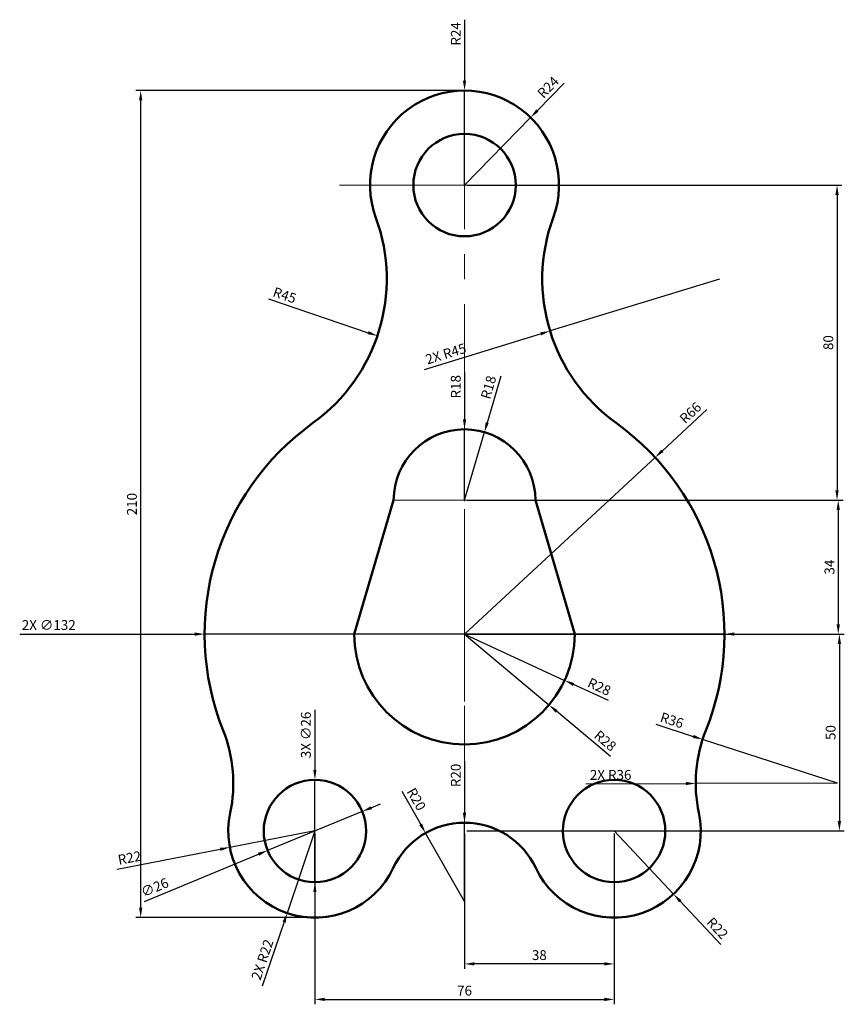
# Model space of a CAD drawing. Units: millimetres. Extents: x 76 to 285, y 1 to 251.
import ezdxf

# ---------------------------------------------------------------- set-up
doc = ezdxf.new("R2010")
doc.units = ezdxf.units.MM
doc.linetypes.add('CENTER', pattern=[50.8, 31.75, -6.35, 6.35, -6.35])
for name, color, linetype, lineweight in [('M-CNTR', 4, 'CENTER', 18), ('M-DIMS', 2, 'Continuous', 25), ('M-OUTL', 7, 'Continuous', 50)]:
    doc.layers.add(name, color=color, linetype=linetype, lineweight=lineweight)
doc.styles.get("Standard").update_dxf_attribs({"font": 'arial.ttf'})
doc.dimstyles.new('ISO-25', dxfattribs={"dimtxt": 2.5, "dimasz": 2.5, "dimexe": 1.25, "dimexo": 0.625, "dimtad": 1, "dimtxsty": 'Standard', "dimcen": 2.5, "dimadec": 0, "dimazin": 0, "dimtfac": 1, "dimtmove": 0, "dimatfit": 3, "dimfxl": 1, "dimarcsym": 0})

# ---------------------------------------------------------------- blocks, each defined once
blk = doc.blocks.new('*D1')
at = {"layer": 'Defpoints', "color": 0, "transparency": 16777216}
for p in [(188.98, 94.94), (188.98, 44.94), (284.18, 44.94)]:
    blk.add_point(p, dxfattribs=at)
at = {"layer": 'M-DIMS', "color": 0, "lineweight": -2, "transparency": 16777216}
for p, q in [((189.6, 94.94), (285.43, 94.94)), ((284.18, 92.44), (284.18, 47.44)), ((189.6, 44.94), (285.43, 44.94))]:
    blk.add_line(p, q, dxfattribs=at)
at = {"layer": 'M-DIMS', "color": 0, "transparency": 16777216}
for points in [[(283.77, 92.44), (284.6, 92.44), (284.18, 94.94)], [(283.77, 47.44), (284.6, 47.44), (284.18, 44.94)]]:
    blk.add_solid(points, dxfattribs=at)
at = {"layer": 'M-DIMS', "color": 0, "transparency": 16777216, "insert": (282.28, 69.94), "char_height": 2.5, "attachment_point": 5, "rotation": 90}
blk.add_mtext('50', dxfattribs=at)
blk = doc.blocks.new('*D2')
at = {"layer": 'Defpoints', "color": 0, "transparency": 16777216}
for p in [(188.98, 128.94), (188.98, 94.94), (283.89, 94.94)]:
    blk.add_point(p, dxfattribs=at)
at = {"layer": 'M-DIMS', "color": 0, "lineweight": -2, "transparency": 16777216}
for p, q in [((189.6, 128.94), (285.14, 128.94)), ((283.89, 126.44), (283.89, 97.44)), ((189.6, 94.94), (285.14, 94.94))]:
    blk.add_line(p, q, dxfattribs=at)
at = {"layer": 'M-DIMS', "color": 0, "transparency": 16777216}
for points in [[(283.47, 126.44), (284.31, 126.44), (283.89, 128.94)], [(283.47, 97.44), (284.31, 97.44), (283.89, 94.94)]]:
    blk.add_solid(points, dxfattribs=at)
at = {"layer": 'M-DIMS', "color": 0, "transparency": 16777216, "insert": (281.99, 111.94), "char_height": 2.5, "attachment_point": 5, "rotation": 90}
blk.add_mtext('34', dxfattribs=at)
blk = doc.blocks.new('*D3')
at = {"layer": 'Defpoints', "color": 0, "transparency": 16777216}
for p in [(188.98, 208.94), (188.98, 128.94), (283.59, 128.94)]:
    blk.add_point(p, dxfattribs=at)
at = {"layer": 'M-DIMS', "color": 0, "lineweight": -2, "transparency": 16777216}
for p, q in [((189.6, 208.94), (284.84, 208.94)), ((283.59, 206.44), (283.59, 131.44)), ((189.6, 128.94), (284.84, 128.94))]:
    blk.add_line(p, q, dxfattribs=at)
at = {"layer": 'M-DIMS', "color": 0, "transparency": 16777216}
for points in [[(283.17, 206.44), (284, 206.44), (283.59, 208.94)], [(283.17, 131.44), (284, 131.44), (283.59, 128.94)]]:
    blk.add_solid(points, dxfattribs=at)
at = {"layer": 'M-DIMS', "color": 0, "transparency": 16777216, "insert": (281.69, 168.94), "char_height": 2.5, "attachment_point": 5, "rotation": 90}
blk.add_mtext('80', dxfattribs=at)
blk = doc.blocks.new('*D4')
at = {"layer": 'Defpoints', "color": 0, "transparency": 16777216}
for p in [(188.98, 94.94), (214.39, 83.19)]:
    blk.add_point(p, dxfattribs=at)
at = {"layer": 'M-DIMS', "color": 0, "lineweight": -2, "transparency": 16777216}
for p, q in [((188.98, 94.94), (214.39, 83.19)), ((225.55, 78.04), (216.66, 82.14))]:
    blk.add_line(p, q, dxfattribs=at)
at = {"layer": 'M-DIMS', "color": 0, "transparency": 16777216}
blk.add_solid([(216.84, 82.52), (216.49, 81.76), (214.39, 83.19)], dxfattribs=at)
at = {"layer": 'M-DIMS', "color": 0, "transparency": 16777216, "insert": (223.07, 81.28), "char_height": 2.5, "attachment_point": 5, "rotation": 335.2019}
blk.add_mtext('R28', dxfattribs=at)
blk = doc.blocks.new('*D5')
at = {"layer": 'Defpoints', "color": 0, "transparency": 16777216}
for p in [(237.39, 139.79), (188.98, 94.94)]:
    blk.add_point(p, dxfattribs=at)
at = {"layer": 'M-DIMS', "color": 0, "lineweight": -2, "transparency": 16777216}
for p, q in [((250.51, 151.95), (239.23, 141.49)), ((188.98, 94.94), (237.39, 139.79))]:
    blk.add_line(p, q, dxfattribs=at)
at = {"layer": 'M-DIMS', "color": 0, "transparency": 16777216}
blk.add_solid([(238.94, 141.79), (239.51, 141.18), (237.39, 139.79)], dxfattribs=at)
at = {"layer": 'M-DIMS', "color": 0, "transparency": 16777216, "insert": (246.57, 150.89), "char_height": 2.5, "attachment_point": 5, "rotation": 42.8138}
blk.add_mtext('R66', dxfattribs=at)
blk = doc.blocks.new('*D6')
at = {"layer": 'Defpoints', "color": 0, "transparency": 16777216}
for p in [(249.45, 68.18), (283.69, 57.08)]:
    blk.add_point(p, dxfattribs=at)
at = {"layer": 'M-DIMS', "color": 0, "lineweight": -2, "transparency": 16777216}
for p, q in [((237.53, 72.04), (247.07, 68.95)), ((283.69, 57.08), (249.45, 68.18))]:
    blk.add_line(p, q, dxfattribs=at)
at = {"layer": 'M-DIMS', "color": 0, "transparency": 16777216}
blk.add_solid([(247.2, 69.35), (246.94, 68.55), (249.45, 68.18)], dxfattribs=at)
at = {"layer": 'M-DIMS', "color": 0, "transparency": 16777216, "insert": (241.56, 72.74), "char_height": 2.5, "attachment_point": 5, "rotation": 342.0409}
blk.add_mtext('R36', dxfattribs=at)
blk = doc.blocks.new('*D7')
at = {"layer": 'Defpoints', "color": 0, "transparency": 16777216}
for p in [(124.23, 185.09), (166.85, 170.67)]:
    blk.add_point(p, dxfattribs=at)
at = {"layer": 'M-DIMS', "color": 0, "lineweight": -2, "transparency": 16777216}
blk.add_line((139.16, 180.04), (164.49, 171.47), dxfattribs=at)
at = {"layer": 'M-DIMS', "color": 0, "transparency": 16777216}
blk.add_solid([(164.62, 171.87), (164.35, 171.08), (166.85, 170.67)], dxfattribs=at)
at = {"layer": 'M-DIMS', "color": 0, "transparency": 16777216, "insert": (143.2, 180.68), "char_height": 2.5, "attachment_point": 5, "rotation": 341.3111}
blk.add_mtext('R45', dxfattribs=at)
blk = doc.blocks.new('*D8')
at = {"layer": 'Defpoints', "color": 0, "transparency": 16777216}
for p in [(162.99, 49.89), (138.96, 39.98)]:
    blk.add_point(p, dxfattribs=at)
at = {"layer": 'M-DIMS', "color": 0, "lineweight": -2, "transparency": 16777216}
for p, q in [((165.3, 50.85), (167.62, 51.8)), ((162.99, 49.89), (138.96, 39.98)), ((107.69, 27.07), (136.65, 39.02))]:
    blk.add_line(p, q, dxfattribs=at)
at = {"layer": 'M-DIMS', "color": 0, "transparency": 16777216}
for points in [[(165.15, 51.23), (165.46, 50.46), (162.99, 49.89)], [(136.49, 39.41), (136.81, 38.64), (138.96, 39.98)]]:
    blk.add_solid(points, dxfattribs=at)
at = {"layer": 'M-DIMS', "color": 0, "transparency": 16777216, "insert": (110.42, 30.33), "char_height": 2.5, "attachment_point": 5, "rotation": 22.4265}
blk.add_mtext('∅26', dxfattribs=at)
blk = doc.blocks.new('*D9')
at = {"layer": 'Defpoints', "color": 0, "transparency": 16777216}
for p in [(150.98, 44.94), (129.37, 40.78)]:
    blk.add_point(p, dxfattribs=at)
at = {"layer": 'M-DIMS', "color": 0, "lineweight": -2, "transparency": 16777216}
for p, q in [((150.98, 44.94), (129.37, 40.78)), ((100.78, 35.27), (126.92, 40.31))]:
    blk.add_line(p, q, dxfattribs=at)
at = {"layer": 'M-DIMS', "color": 0, "transparency": 16777216}
blk.add_solid([(126.84, 40.71), (127, 39.9), (129.37, 40.78)], dxfattribs=at)
at = {"layer": 'M-DIMS', "color": 0, "transparency": 16777216, "insert": (103.96, 37.8), "char_height": 2.5, "attachment_point": 5, "rotation": 10.8931}
blk.add_mtext('R22', dxfattribs=at)
blk = doc.blocks.new('*D10')
at = {"layer": 'Defpoints', "color": 0, "transparency": 16777216}
for p in [(205.75, 226.1), (188.98, 208.94)]:
    blk.add_point(p, dxfattribs=at)
at = {"layer": 'M-DIMS', "color": 0, "lineweight": -2, "transparency": 16777216}
for p, q in [((214.29, 234.83), (207.5, 227.89)), ((188.98, 208.94), (205.75, 226.1))]:
    blk.add_line(p, q, dxfattribs=at)
at = {"layer": 'M-DIMS', "color": 0, "transparency": 16777216}
blk.add_solid([(207.2, 228.18), (207.8, 227.59), (205.75, 226.1)], dxfattribs=at)
at = {"layer": 'M-DIMS', "color": 0, "transparency": 16777216, "insert": (210.43, 233.57), "char_height": 2.5, "attachment_point": 5, "rotation": 45.6505}
blk.add_mtext('R24', dxfattribs=at)
blk = doc.blocks.new('*D11')
at = {"layer": 'Defpoints', "color": 0, "transparency": 16777216}
for p in [(226.98, 44.94), (242.05, 28.91)]:
    blk.add_point(p, dxfattribs=at)
at = {"layer": 'M-DIMS', "color": 0, "lineweight": -2, "transparency": 16777216}
for p, q in [((226.98, 44.94), (242.05, 28.91)), ((254.07, 16.14), (243.77, 27.09))]:
    blk.add_line(p, q, dxfattribs=at)
at = {"layer": 'M-DIMS', "color": 0, "transparency": 16777216}
blk.add_solid([(244.07, 27.38), (243.46, 26.81), (242.05, 28.91)], dxfattribs=at)
at = {"layer": 'M-DIMS', "color": 0, "transparency": 16777216, "insert": (252.97, 20.05), "char_height": 2.5, "attachment_point": 5, "rotation": 313.2557}
blk.add_mtext('R22', dxfattribs=at)
blk = doc.blocks.new('*D12')
at = {"layer": 'Defpoints', "color": 0, "transparency": 16777216}
for p in [(150.98, 44.94), (226.98, 44.94), (226.98, 2.18)]:
    blk.add_point(p, dxfattribs=at)
at = {"layer": 'M-DIMS', "color": 0, "lineweight": -2, "transparency": 16777216}
for p, q in [((150.98, 44.31), (150.98, 0.93)), ((226.98, 44.31), (226.98, 0.93)), ((153.48, 2.18), (224.48, 2.18))]:
    blk.add_line(p, q, dxfattribs=at)
at = {"layer": 'M-DIMS', "color": 0, "transparency": 16777216}
for points in [[(153.48, 2.6), (153.48, 1.76), (150.98, 2.18)], [(224.48, 2.6), (224.48, 1.76), (226.98, 2.18)]]:
    blk.add_solid(points, dxfattribs=at)
at = {"layer": 'M-DIMS', "color": 0, "transparency": 16777216, "insert": (188.98, 4.08), "char_height": 2.5, "attachment_point": 5}
blk.add_mtext('76', dxfattribs=at)
blk = doc.blocks.new('*D13')
at = {"layer": 'Defpoints', "color": 0, "transparency": 16777216}
for p in [(188.98, 44.94), (226.98, 44.94), (188.98, 11.19)]:
    blk.add_point(p, dxfattribs=at)
at = {"layer": 'M-DIMS', "color": 0, "lineweight": -2, "transparency": 16777216}
for p, q in [((188.98, 44.31), (188.98, 9.94)), ((226.98, 44.31), (226.98, 9.94)), ((224.48, 11.19), (191.48, 11.19))]:
    blk.add_line(p, q, dxfattribs=at)
at = {"layer": 'M-DIMS', "color": 0, "transparency": 16777216}
for points in [[(191.48, 11.61), (191.48, 10.78), (188.98, 11.19)], [(224.48, 11.61), (224.48, 10.78), (226.98, 11.19)]]:
    blk.add_solid(points, dxfattribs=at)
at = {"layer": 'M-DIMS', "color": 0, "transparency": 16777216, "insert": (207.98, 13.1), "char_height": 2.5, "attachment_point": 5}
blk.add_mtext('38', dxfattribs=at)
blk = doc.blocks.new('*D14')
at = {"layer": 'Defpoints', "color": 0, "transparency": 16777216}
for p in [(179.08, 44.42), (188.98, 27.05)]:
    blk.add_point(p, dxfattribs=at)
at = {"layer": 'M-DIMS', "color": 0, "lineweight": -2, "transparency": 16777216}
for p, q in [((173.03, 55.04), (177.84, 46.6)), ((188.98, 27.05), (179.08, 44.42))]:
    blk.add_line(p, q, dxfattribs=at)
at = {"layer": 'M-DIMS', "color": 0, "transparency": 16777216}
blk.add_solid([(178.2, 46.8), (177.48, 46.39), (179.08, 44.42)], dxfattribs=at)
at = {"layer": 'M-DIMS', "color": 0, "transparency": 16777216, "insert": (176.47, 52.85), "char_height": 2.5, "attachment_point": 5, "rotation": 299.6684}
blk.add_mtext('R20', dxfattribs=at)
blk = doc.blocks.new('*D15')
at = {"layer": 'Defpoints', "color": 0, "transparency": 16777216}
for p in [(194.04, 146.21), (188.98, 128.94)]:
    blk.add_point(p, dxfattribs=at)
at = {"layer": 'M-DIMS', "color": 0, "lineweight": -2, "transparency": 16777216}
for p, q in [((198.21, 160.44), (194.74, 148.61)), ((188.98, 128.94), (194.04, 146.21))]:
    blk.add_line(p, q, dxfattribs=at)
at = {"layer": 'M-DIMS', "color": 0, "transparency": 16777216}
blk.add_solid([(194.34, 148.73), (195.14, 148.49), (194.04, 146.21)], dxfattribs=at)
at = {"layer": 'M-DIMS', "color": 0, "transparency": 16777216, "insert": (195.37, 157.51), "char_height": 2.5, "attachment_point": 5, "rotation": 73.667}
blk.add_mtext('R18', dxfattribs=at)
blk = doc.blocks.new('THRU-HOLE-D26')
blk.add_circle((13, 13), 13)
blk = doc.blocks.new('*D17')
at = {"layer": 'Defpoints', "color": 0, "transparency": 16777216}
for p in [(106.73, 232.94), (188.98, 232.94), (151.95, 22.95)]:
    blk.add_point(p, dxfattribs=at)
at = {"layer": 'M-DIMS', "color": 0, "lineweight": -2, "transparency": 16777216}
for p, q in [((188.35, 232.94), (105.48, 232.94)), ((106.73, 25.45), (106.73, 230.44)), ((151.33, 22.95), (105.48, 22.95))]:
    blk.add_line(p, q, dxfattribs=at)
at = {"layer": 'M-DIMS', "color": 0, "transparency": 16777216}
for points in [[(106.32, 230.44), (107.15, 230.44), (106.73, 232.94)], [(106.32, 25.45), (107.15, 25.45), (106.73, 22.95)]]:
    blk.add_solid(points, dxfattribs=at)
at = {"layer": 'M-DIMS', "color": 0, "transparency": 16777216, "insert": (104.83, 127.94), "char_height": 2.5, "attachment_point": 5, "rotation": 90}
blk.add_mtext('210', dxfattribs=at)
blk = doc.blocks.new('*D18')
at = {"layer": 'Defpoints', "color": 0, "transparency": 16777216}
for p in [(122.98, 94.93), (254.98, 94.94)]:
    blk.add_point(p, dxfattribs=at)
at = {"layer": 'M-DIMS', "color": 0, "lineweight": -2, "transparency": 16777216}
for p, q in [((76, 94.93), (120.48, 94.93)), ((254.98, 94.94), (122.98, 94.93)), ((257.48, 94.94), (259.98, 94.94))]:
    blk.add_line(p, q, dxfattribs=at)
at = {"layer": 'M-DIMS', "color": 0, "transparency": 16777216}
for points in [[(120.48, 95.35), (120.48, 94.52), (122.98, 94.93)], [(257.48, 95.35), (257.48, 94.52), (254.98, 94.94)]]:
    blk.add_solid(points, dxfattribs=at)
at = {"layer": 'M-DIMS', "color": 0, "transparency": 16777216, "insert": (83.38, 96.91), "char_height": 2.5, "attachment_point": 5, "rotation": 0.0002}
blk.add_mtext('2X ∅132', dxfattribs=at)
blk = doc.blocks.new('*D19')
at = {"layer": 'Defpoints', "color": 0, "transparency": 16777216}
for p in [(150.98, 57.94), (150.98, 31.94)]:
    blk.add_point(p, dxfattribs=at)
at = {"layer": 'M-DIMS', "color": 0, "lineweight": -2, "transparency": 16777216}
for p, q in [((150.98, 75.72), (150.98, 60.44)), ((150.98, 31.94), (150.98, 57.94)), ((150.98, 29.44), (150.98, 26.94))]:
    blk.add_line(p, q, dxfattribs=at)
at = {"layer": 'M-DIMS', "color": 0, "transparency": 16777216}
for points in [[(150.56, 60.44), (151.39, 60.44), (150.98, 57.94)], [(150.56, 29.44), (151.39, 29.44), (150.98, 31.94)]]:
    blk.add_solid(points, dxfattribs=at)
at = {"layer": 'M-DIMS', "color": 0, "transparency": 16777216, "insert": (149.01, 69.33), "char_height": 2.5, "attachment_point": 5, "rotation": 89.9991}
blk.add_mtext('3X ∅26', dxfattribs=at)
blk = doc.blocks.new('*D20')
at = {"layer": 'Defpoints', "color": 0, "transparency": 16777216}
for p in [(188.98, 232.94), (188.98, 208.94)]:
    blk.add_point(p, dxfattribs=at)
at = {"layer": 'M-DIMS', "color": 0, "lineweight": -2, "transparency": 16777216}
for p, q in [((188.98, 250.94), (188.98, 235.44)), ((188.98, 208.94), (188.98, 232.94))]:
    blk.add_line(p, q, dxfattribs=at)
at = {"layer": 'M-DIMS', "color": 0, "transparency": 16777216}
blk.add_solid([(188.56, 235.44), (189.39, 235.44), (188.98, 232.94)], dxfattribs=at)
at = {"layer": 'M-DIMS', "color": 0, "transparency": 16777216, "insert": (187.1, 247.34), "char_height": 2.5, "attachment_point": 5, "rotation": 89.9995}
blk.add_mtext('R24', dxfattribs=at)
blk = doc.blocks.new('*D21')
at = {"layer": 'Defpoints', "color": 0, "transparency": 16777216}
for p in [(253.73, 185.09), (210.7, 171.9)]:
    blk.add_point(p, dxfattribs=at)
at = {"layer": 'M-DIMS', "color": 0, "lineweight": -2, "transparency": 16777216}
for p, q in [((253.73, 185.09), (210.7, 171.9)), ((178.84, 162.13), (208.31, 171.17))]:
    blk.add_line(p, q, dxfattribs=at)
at = {"layer": 'M-DIMS', "color": 0, "transparency": 16777216}
blk.add_solid([(208.19, 171.56), (208.44, 170.77), (210.7, 171.9)], dxfattribs=at)
at = {"layer": 'M-DIMS', "color": 0, "transparency": 16777216, "insert": (184.33, 165.8), "char_height": 2.5, "attachment_point": 5, "rotation": 17.0501}
blk.add_mtext('2X R45', dxfattribs=at)
blk = doc.blocks.new('*D22')
at = {"layer": 'Defpoints', "color": 0, "transparency": 16777216}
for p in [(247.69, 57), (283.69, 57.08)]:
    blk.add_point(p, dxfattribs=at)
at = {"layer": 'M-DIMS', "color": 0, "lineweight": -2, "transparency": 16777216}
for p, q in [((219.77, 56.94), (245.19, 56.99)), ((283.69, 57.08), (247.69, 57))]:
    blk.add_line(p, q, dxfattribs=at)
at = {"layer": 'M-DIMS', "color": 0, "transparency": 16777216}
blk.add_solid([(245.19, 57.41), (245.19, 56.58), (247.69, 57)], dxfattribs=at)
at = {"layer": 'M-DIMS', "color": 0, "transparency": 16777216, "insert": (226.09, 58.86), "char_height": 2.5, "attachment_point": 5, "rotation": 0.1249}
blk.add_mtext('2X R36', dxfattribs=at)
blk = doc.blocks.new('*D23')
at = {"layer": 'Defpoints', "color": 0, "transparency": 16777216}
for p in [(150.98, 44.94), (143.94, 24.09)]:
    blk.add_point(p, dxfattribs=at)
at = {"layer": 'M-DIMS', "color": 0, "lineweight": -2, "transparency": 16777216}
for p, q in [((150.98, 44.94), (143.94, 24.09)), ((137.71, 5.61), (143.14, 21.72))]:
    blk.add_line(p, q, dxfattribs=at)
at = {"layer": 'M-DIMS', "color": 0, "transparency": 16777216}
blk.add_solid([(142.75, 21.85), (143.54, 21.59), (143.94, 24.09)], dxfattribs=at)
at = {"layer": 'M-DIMS', "color": 0, "transparency": 16777216, "insert": (137.94, 12.18), "char_height": 2.5, "attachment_point": 5, "rotation": 71.3541}
blk.add_mtext('2X R22', dxfattribs=at)
blk = doc.blocks.new('*D24')
at = {"layer": 'Defpoints', "color": 0, "transparency": 16777216}
for p in [(188.98, 47.05), (188.98, 27.05)]:
    blk.add_point(p, dxfattribs=at)
at = {"layer": 'M-DIMS', "color": 0, "lineweight": -2, "transparency": 16777216}
for p, q in [((188.98, 62.65), (188.98, 49.55)), ((188.98, 27.05), (188.98, 47.05))]:
    blk.add_line(p, q, dxfattribs=at)
at = {"layer": 'M-DIMS', "color": 0, "transparency": 16777216}
blk.add_solid([(188.56, 49.55), (189.39, 49.55), (188.98, 47.05)], dxfattribs=at)
at = {"layer": 'M-DIMS', "color": 0, "transparency": 16777216, "insert": (187.08, 59.05), "char_height": 2.5, "attachment_point": 5, "rotation": 89.9994}
blk.add_mtext('R20', dxfattribs=at)
blk = doc.blocks.new('*D25')
at = {"layer": 'Defpoints', "color": 0, "transparency": 16777216}
for p in [(188.98, 94.94), (210.43, 76.94)]:
    blk.add_point(p, dxfattribs=at)
at = {"layer": 'M-DIMS', "color": 0, "lineweight": -2, "transparency": 16777216}
for p, q in [((188.98, 94.94), (210.43, 76.94)), ((226.07, 63.82), (212.34, 75.33))]:
    blk.add_line(p, q, dxfattribs=at)
at = {"layer": 'M-DIMS', "color": 0, "transparency": 16777216}
blk.add_solid([(212.61, 75.65), (212.08, 75.01), (210.43, 76.94)], dxfattribs=at)
at = {"layer": 'M-DIMS', "color": 0, "transparency": 16777216, "insert": (224.52, 67.6), "char_height": 2.5, "attachment_point": 5, "rotation": 320.0096}
blk.add_mtext('R28', dxfattribs=at)
blk = doc.blocks.new('*D26')
at = {"layer": 'Defpoints', "color": 0, "transparency": 16777216}
for p in [(188.98, 146.94), (188.98, 128.94)]:
    blk.add_point(p, dxfattribs=at)
at = {"layer": 'M-DIMS', "color": 0, "lineweight": -2, "transparency": 16777216}
for p, q in [((188.98, 161.35), (188.98, 149.44)), ((188.98, 128.94), (188.98, 146.94))]:
    blk.add_line(p, q, dxfattribs=at)
at = {"layer": 'M-DIMS', "color": 0, "transparency": 16777216}
blk.add_solid([(188.56, 149.44), (189.39, 149.44), (188.98, 146.94)], dxfattribs=at)
at = {"layer": 'M-DIMS', "color": 0, "transparency": 16777216, "insert": (187.08, 157.74), "char_height": 2.5, "attachment_point": 5, "rotation": 89.9994}
blk.add_mtext('R18', dxfattribs=at)

msp = doc.modelspace()

# ---------------------------------------------------------------- linework, layer by layer
at = {"layer": 'M-CNTR'}
for p, q in [((188.977, 146.935), (188.977, 232.935)), ((188.977, 208.935), (152.766, 208.935)), ((188.977, 208.935), (240.425, 208.935)), ((188.977, 27.047), (188.977, 146.935)), ((188.977, 128.935), (188.977, 146.935)), ((188.977, 128.935), (170.977, 128.935)), ((188.977, 94.935), (188.977, 128.935)), ((188.977, 128.935), (195.491, 128.935)), ((195.491, 128.935), (206.977, 128.935)), ((188.977, 94.935), (160.977, 94.935)), ((188.977, 44.935), (188.977, 94.935)), ((188.977, 94.935), (203.425, 94.935)), ((203.425, 94.935), (216.977, 94.935))]:
    msp.add_line(p, q, dxfattribs=at)
at = {"layer": 'M-OUTL'}
for p, q in [((160.977, 94.935), (170.977, 128.935)), ((216.977, 94.935), (206.977, 128.935))]:
    msp.add_line(p, q, dxfattribs=at)
for centre, radius, start, end in [((188.977, 208.935), 24, 339.78537, 200.21463), ((124.227, 185.093), 45, 305.68529, 20.21463), ((253.727, 185.093), 45, 159.78537, 234.31471), ((188.977, 94.935), 66, 125.68529, 201.78632), ((188.977, 94.935), 66, 338.21368, 54.31471), ((188.977, 128.935), 18, 0, 180), ((188.977, 94.935), 28, 180, 0), ((94.262, 57.078), 36, 347.91494, 21.78632), ((283.691, 57.078), 36, 158.21368, 192.08506), ((150.977, 44.935), 22, 167.91494, 334.79123), ((226.977, 44.935), 22, 205.20877, 12.08506), ((188.977, 27.047), 20, 25.20877, 154.79123)]:
    msp.add_arc(centre, radius, start, end, dxfattribs=at)

# ---------------------------------------------------------------- block references
for p in [(175.977, 195.935), (137.977, 31.935), (213.977, 31.935)]:
    msp.add_blockref('THRU-HOLE-D26', p, dxfattribs=at)

# ---------------------------------------------------------------- dimensions: what is measured, and where the dimension line sits
at = {"layer": 'M-DIMS'}
for center, mpoint, override, picture, middle in [((188.977, 208.935), (188.977, 232.935), {"dimdec": 0, "dimlfac": 1, "dimrnd": 0, "dimzin": 0, "dimdsep": 46, "dimlunit": 2}, '*D20', (188.977, 247.335)), ((124.227, 185.093), (166.854, 170.674), {"dimclrd": 0, "dimclre": 0, "dimclrt": 0}, '*D7', (142.592, 178.881)), ((188.977, 128.935), (188.977, 146.935), {"dimdec": 0, "dimlfac": 1, "dimrnd": 0, "dimzin": 0, "dimdsep": 46, "dimlunit": 2}, '*D26', (188.977, 157.735)), ((188.977, 128.935), (194.039, 146.209), {"dimclrd": 0, "dimclre": 0, "dimclrt": 0}, '*D15', (197.193, 156.972)), ((188.977, 94.935), (237.392, 139.79), {"dimclrd": 0, "dimclre": 0, "dimclrt": 0}, '*D5', (247.864, 149.492)), ((188.977, 94.935), (214.395, 83.191), {"dimclrd": 0, "dimclre": 0, "dimclrt": 0}, '*D4', (222.27, 79.553)), ((188.977, 94.935), (210.429, 76.941), {"dimdec": 0, "dimlfac": 1, "dimrnd": 0, "dimzin": 0, "dimdsep": 46, "dimlunit": 2}, '*D25', (223.3, 66.144)), ((283.691, 57.078), (249.445, 68.179), {"dimclrd": 0, "dimclre": 0, "dimclrt": 0}, '*D6', (240.969, 70.926)), ((188.977, 27.047), (188.977, 47.047), {"dimdec": 0, "dimlfac": 1, "dimrnd": 0, "dimzin": 0, "dimdsep": 46, "dimlunit": 2}, '*D24', (188.977, 59.047)), ((150.977, 44.935), (129.373, 40.778), {"dimclrd": 0, "dimclre": 0, "dimclrt": 0}, '*D9', (104.311, 35.955)), ((226.977, 44.935), (242.052, 28.913), {"dimclrd": 0, "dimclre": 0, "dimclrt": 0}, '*D11', (251.602, 18.763))]:
    dim = msp.add_radius_dim(center=center, mpoint=mpoint, dimstyle='ISO-25', override=override, dxfattribs=at)
    dim.commit()
    dim.dimension.update_dxf_attribs({"geometry": picture, "text_midpoint": middle, "dimtype": 164})
for center, mpoint, picture, middle in [((188.977, 208.935), (205.754, 226.097), '*D10', (210.426, 233.566)), ((188.977, 27.047), (179.077, 44.425), '*D14', (176.469, 52.845))]:
    dim = msp.add_radius_dim(center=center, mpoint=mpoint, dimstyle='ISO-25', override={"dimclrd": 0, "dimclre": 0, "dimclrt": 0}, dxfattribs=at)
    dim.commit()
    dim.dimension.update_dxf_attribs({"geometry": picture, "text_midpoint": middle})
for base, p1, p2, override, picture, middle in [((106.734, 232.935), (151.95, 22.953), (188.977, 232.935), {"dimdec": 0, "dimlfac": 1, "dimrnd": 0, "dimzin": 0, "dimdsep": 46, "dimlunit": 2}, '*D17', (104.833, 127.944)), ((283.588, 128.935), (188.977, 208.935), (188.977, 128.935), {"dimclrd": 0, "dimclre": 0, "dimclrt": 0}, '*D3', (281.687, 168.935)), ((283.89, 94.935), (188.977, 128.935), (188.977, 94.935), {"dimclrd": 0, "dimclre": 0, "dimclrt": 0}, '*D2', (281.987, 111.935)), ((284.183, 44.935), (188.977, 94.935), (188.977, 44.935), {"dimclrd": 0, "dimclre": 0, "dimclrt": 0}, '*D1', (282.282, 69.935))]:
    dim = msp.add_linear_dim(base=base, p1=p1, p2=p2, angle=90, dimstyle='ISO-25', override=override, dxfattribs=at)
    dim.commit()
    dim.dimension.update_dxf_attribs({"geometry": picture, "text_midpoint": middle})
for center, mpoint, picture, middle in [((253.727, 185.093), (210.705, 171.899), '*D21', (184.891, 163.982)), ((283.691, 57.078), (247.691, 57), '*D22', (226.092, 56.953)), ((150.977, 44.935), (143.943, 24.09), '*D23', (139.723, 11.583))]:
    dim = msp.add_radius_dim(center=center, mpoint=mpoint, text='2X <>', dimstyle='ISO-25', override={"dimdec": 0, "dimlfac": 1, "dimrnd": 0, "dimzin": 0, "dimdsep": 46, "dimlunit": 2}, dxfattribs=at)
    dim.commit()
    dim.dimension.update_dxf_attribs({"geometry": picture, "text_midpoint": middle, "dimtype": 164})
dim = msp.add_diameter_dim_2p(p1=(254.977, 94.936), p2=(122.977, 94.935), text='2X <>', dimstyle='ISO-25', override={"dimdec": 0, "dimlfac": 1, "dimrnd": 0, "dimzin": 0, "dimdsep": 46, "dimlunit": 2}, dxfattribs=at)
dim.commit()
dim.dimension.update_dxf_attribs({"geometry": '*D18', "text_midpoint": (83.377, 94.935), "dimtype": 163})
dim = msp.add_diameter_dim_2p(p1=(150.977, 31.935), p2=(150.977, 57.935), text='3X <>', dimstyle='ISO-25', override={"dimdec": 0, "dimlfac": 1, "dimrnd": 0, "dimzin": 0, "dimdsep": 46, "dimlunit": 2}, dxfattribs=at)
dim.commit()
dim.dimension.update_dxf_attribs({"geometry": '*D19', "text_midpoint": (150.977, 69.329)})
dim = msp.add_diameter_dim_2p(p1=(162.994, 49.895), p2=(138.96, 39.976), dimstyle='ISO-25', override={"dimclrd": 0, "dimclre": 0, "dimclrt": 0}, dxfattribs=at)
dim.commit()
dim.dimension.update_dxf_attribs({"geometry": '*D8', "text_midpoint": (111.176, 28.509), "dimtype": 163})
for base, p1, p2, picture, middle in [((226.977, 2.18), (150.977, 44.935), (226.977, 44.935), '*D12', (188.977, 4.082)), ((188.977, 11.195), (226.977, 44.935), (188.977, 44.935), '*D13', (207.977, 13.097))]:
    dim = msp.add_linear_dim(base=base, p1=p1, p2=p2, dimstyle='ISO-25', override={"dimclrd": 0, "dimclre": 0, "dimclrt": 0}, dxfattribs=at)
    dim.commit()
    dim.dimension.update_dxf_attribs({"geometry": picture, "text_midpoint": middle})

doc.saveas('drawing.dxf')
